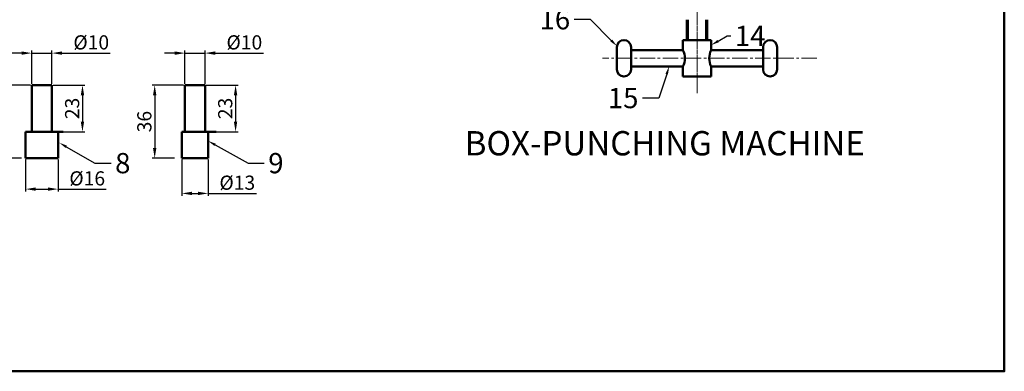
# Model space of a CAD drawing. Units: millimetres. Extents: x 434 to 1535, y -197 to 318.
# Tile 8 of 9: x 1049 to 1535, y -197 to -24. Entities that reach past the tile are written whole.
import ezdxf
from ezdxf import colors
from ezdxf.entities.mleader import LeaderData, LeaderLine
from ezdxf.math import Vec2, Vec3

# ---------------------------------------------------------------- set-up
doc = ezdxf.new("R2010")
doc.units = ezdxf.units.MM
doc.header["$LTSCALE"] = 0.4
doc.linetypes.add('CENTER2', pattern=[28.575, 19.05, -3.175, 3.175, -3.175])
for name, color, linetype, lineweight in [('M-CNTR', 1, 'CENTER2', 18), ('M-DIMS', 2, 'Continuous', 25), ('M-OUTL', 7, 'Continuous', 50), ('M-TEXT', 3, 'Continuous', 25)]:
    doc.layers.add(name, color=color, linetype=linetype, lineweight=lineweight)
doc.styles.get("Standard").update_dxf_attribs({"font": 'arial.ttf'})
doc.dimstyles.new('ISO-25', dxfattribs={"dimtxt": 7, "dimasz": 5, "dimexe": 1.25, "dimexo": 0.625, "dimtad": 1, "dimtoh": 1, "dimdec": 0, "dimtxsty": 'Standard', "dimcen": 2.5, "dimadec": 0, "dimazin": 0, "dimtfac": 1, "dimtdec": 0, "dimtmove": 0, "dimatfit": 3, "dimfxl": 1, "dimarcsym": 0})

# ---------------------------------------------------------------- blocks, each defined once
blk = doc.blocks.new('*U4')
at = {"layer": 'M-CNTR', "color": 0, "transparency": 16777216}
for p, q in [((0, 7), (0, 38.5)), ((-38.5, 0), (-7, 0)), ((7, 0), (73.2, 0)), ((0, -198.75), (0, -7))]:
    blk.add_line(p, q, dxfattribs=at)
at = {"layer": 'M-CNTR', "color": 0, "linetype": 'Continuous', "transparency": 16777216}
for p, q in [((-3.5, 0), (3.5, 0)), ((0, -3.5), (0, 3.5))]:
    blk.add_line(p, q, dxfattribs=at)
blk = doc.blocks.new('*U80')
at = {"layer": 'M-CNTR', "color": 0, "transparency": 16777216}
blk.add_line((0, -17.2), (0, 69.52), dxfattribs=at)
blk = doc.blocks.new('*U81')
at = {"layer": 'M-CNTR', "color": 0, "transparency": 16777216}
blk.add_line((59.26, 0), (-46.77, 0), dxfattribs=at)
blk = doc.blocks.new('*D120')
at = {"layer": 'Defpoints', "color": 0, "ltscale": 0.4, "transparency": 16777216}
for p in [(1064.56, -40.42), (1054.56, -56.24), (1064.56, -56.24)]:
    blk.add_point(p, dxfattribs=at)
at = {"layer": 'M-DIMS', "color": 0, "lineweight": -2, "ltscale": 0.4, "transparency": 16777216}
for p, q in [((1049.56, -40.42), (1044.56, -40.42)), ((1054.56, -55.61), (1054.56, -39.17)), ((1054.56, -40.42), (1064.56, -40.42)), ((1064.56, -55.61), (1064.56, -39.17)), ((1069.56, -40.42), (1093.43, -40.42))]:
    blk.add_line(p, q, dxfattribs=at)
at = {"layer": 'M-DIMS', "color": 0, "ltscale": 0.4, "transparency": 16777216}
for points in [[(1049.56, -39.59), (1049.56, -41.26), (1054.56, -40.42)], [(1069.56, -39.59), (1069.56, -41.26), (1064.56, -40.42)]]:
    blk.add_solid(points, dxfattribs=at)
at = {"layer": 'M-DIMS', "color": 0, "ltscale": 0.4, "transparency": 16777216, "insert": (1083.99, -36.03), "char_height": 7, "attachment_point": 5}
blk.add_mtext('%%C10', dxfattribs=at)
blk = doc.blocks.new('*D121')
at = {"layer": 'Defpoints', "color": 0, "ltscale": 0.4, "transparency": 16777216}
for p in [(1064.56, -56.24), (1064.56, -79.24), (1079.65, -79.24)]:
    blk.add_point(p, dxfattribs=at)
at = {"layer": 'M-DIMS', "color": 0, "lineweight": -2, "ltscale": 0.4, "transparency": 16777216}
for p, q in [((1065.18, -56.24), (1080.9, -56.24)), ((1079.65, -61.24), (1079.65, -74.24)), ((1065.18, -79.24), (1080.9, -79.24))]:
    blk.add_line(p, q, dxfattribs=at)
at = {"layer": 'M-DIMS', "color": 0, "ltscale": 0.4, "transparency": 16777216}
for points in [[(1078.82, -61.24), (1080.48, -61.24), (1079.65, -56.24)], [(1078.82, -74.24), (1080.48, -74.24), (1079.65, -79.24)]]:
    blk.add_solid(points, dxfattribs=at)
at = {"layer": 'M-DIMS', "color": 0, "ltscale": 0.4, "transparency": 16777216, "insert": (1075.45, -67.74), "char_height": 7, "attachment_point": 5, "rotation": 90}
blk.add_mtext('23', dxfattribs=at)
blk = doc.blocks.new('*D119')
at = {"layer": 'Defpoints', "color": 0, "ltscale": 0.4, "transparency": 16777216}
for p in [(1054.56, -56.24), (1039.66, -92.24), (1050.06, -92.24)]:
    blk.add_point(p, dxfattribs=at)
at = {"layer": 'M-DIMS', "color": 0, "lineweight": -2, "ltscale": 0.4, "transparency": 16777216}
for p, q in [((1053.93, -56.24), (1038.41, -56.24)), ((1039.66, -61.24), (1039.66, -87.24)), ((1049.43, -92.24), (1038.41, -92.24))]:
    blk.add_line(p, q, dxfattribs=at)
at = {"layer": 'M-DIMS', "color": 0, "ltscale": 0.4, "transparency": 16777216}
for points in [[(1038.83, -61.24), (1040.49, -61.24), (1039.66, -56.24)], [(1038.83, -87.24), (1040.49, -87.24), (1039.66, -92.24)]]:
    blk.add_solid(points, dxfattribs=at)
at = {"layer": 'M-DIMS', "color": 0, "ltscale": 0.4, "transparency": 16777216, "insert": (1035.46, -74.24), "char_height": 7, "attachment_point": 5, "rotation": 90}
blk.add_mtext('36', dxfattribs=at)
blk = doc.blocks.new('*D123')
at = {"layer": 'Defpoints', "color": 0, "ltscale": 0.4, "transparency": 16777216}
for p in [(1140.27, -40.42), (1130.27, -56.24), (1140.27, -56.24)]:
    blk.add_point(p, dxfattribs=at)
at = {"layer": 'M-DIMS', "color": 0, "lineweight": -2, "ltscale": 0.4, "transparency": 16777216}
for p, q in [((1125.27, -40.42), (1120.27, -40.42)), ((1130.27, -55.61), (1130.27, -39.17)), ((1130.27, -40.42), (1140.27, -40.42)), ((1140.27, -55.61), (1140.27, -39.17)), ((1145.27, -40.42), (1169.13, -40.42))]:
    blk.add_line(p, q, dxfattribs=at)
at = {"layer": 'M-DIMS', "color": 0, "ltscale": 0.4, "transparency": 16777216}
for points in [[(1125.27, -39.59), (1125.27, -41.26), (1130.27, -40.42)], [(1145.27, -39.59), (1145.27, -41.26), (1140.27, -40.42)]]:
    blk.add_solid(points, dxfattribs=at)
at = {"layer": 'M-DIMS', "color": 0, "ltscale": 0.4, "transparency": 16777216, "insert": (1159.7, -36.03), "char_height": 7, "attachment_point": 5}
blk.add_mtext('%%C10', dxfattribs=at)
blk = doc.blocks.new('*D124')
at = {"layer": 'Defpoints', "color": 0, "ltscale": 0.4, "transparency": 16777216}
for p in [(1140.27, -56.24), (1140.27, -79.24), (1155.36, -79.24)]:
    blk.add_point(p, dxfattribs=at)
at = {"layer": 'M-DIMS', "color": 0, "lineweight": -2, "ltscale": 0.4, "transparency": 16777216}
for p, q in [((1140.89, -56.24), (1156.61, -56.24)), ((1155.36, -61.24), (1155.36, -74.24)), ((1140.89, -79.24), (1156.61, -79.24))]:
    blk.add_line(p, q, dxfattribs=at)
at = {"layer": 'M-DIMS', "color": 0, "ltscale": 0.4, "transparency": 16777216}
for points in [[(1154.52, -61.24), (1156.19, -61.24), (1155.36, -56.24)], [(1154.52, -74.24), (1156.19, -74.24), (1155.36, -79.24)]]:
    blk.add_solid(points, dxfattribs=at)
at = {"layer": 'M-DIMS', "color": 0, "ltscale": 0.4, "transparency": 16777216, "insert": (1151.15, -67.74), "char_height": 7, "attachment_point": 5, "rotation": 90}
blk.add_mtext('23', dxfattribs=at)
blk = doc.blocks.new('*D122')
at = {"layer": 'Defpoints', "color": 0, "ltscale": 0.4, "transparency": 16777216}
for p in [(1130.27, -56.24), (1115.37, -92.24), (1125.77, -92.24)]:
    blk.add_point(p, dxfattribs=at)
at = {"layer": 'M-DIMS', "color": 0, "lineweight": -2, "ltscale": 0.4, "transparency": 16777216}
for p, q in [((1129.64, -56.24), (1114.12, -56.24)), ((1115.37, -61.24), (1115.37, -87.24)), ((1125.14, -92.24), (1114.12, -92.24))]:
    blk.add_line(p, q, dxfattribs=at)
at = {"layer": 'M-DIMS', "color": 0, "ltscale": 0.4, "transparency": 16777216}
for points in [[(1114.53, -61.24), (1116.2, -61.24), (1115.37, -56.24)], [(1114.53, -87.24), (1116.2, -87.24), (1115.37, -92.24)]]:
    blk.add_solid(points, dxfattribs=at)
at = {"layer": 'M-DIMS', "color": 0, "ltscale": 0.4, "transparency": 16777216, "insert": (1111.16, -74.24), "char_height": 7, "attachment_point": 5, "rotation": 90}
blk.add_mtext('36', dxfattribs=at)
blk = doc.blocks.new('*D125')
at = {"layer": 'Defpoints', "color": 0, "ltscale": 0.4, "transparency": 16777216}
for p in [(1051.56, -92.24), (1067.56, -92.24), (1067.56, -107.55)]:
    blk.add_point(p, dxfattribs=at)
at = {"layer": 'M-DIMS', "color": 0, "lineweight": -2, "ltscale": 0.4, "transparency": 16777216}
for p, q in [((1051.56, -92.86), (1051.56, -108.8)), ((1067.56, -92.86), (1067.56, -108.8)), ((1056.56, -107.55), (1062.56, -107.55)), ((1067.56, -107.55), (1091.45, -107.55))]:
    blk.add_line(p, q, dxfattribs=at)
at = {"layer": 'M-DIMS', "color": 0, "ltscale": 0.4, "transparency": 16777216}
for points in [[(1056.56, -106.72), (1056.56, -108.39), (1051.56, -107.55)], [(1062.56, -106.72), (1062.56, -108.39), (1067.56, -107.55)]]:
    blk.add_solid(points, dxfattribs=at)
at = {"layer": 'M-DIMS', "color": 0, "ltscale": 0.4, "transparency": 16777216, "insert": (1082, -103.16), "char_height": 7, "attachment_point": 5}
blk.add_mtext('%%C16', dxfattribs=at)
blk = doc.blocks.new('*D126')
at = {"layer": 'Defpoints', "color": 0, "ltscale": 0.4, "transparency": 16777216}
for p in [(1128.77, -92.24), (1141.77, -92.24), (1141.77, -109.69)]:
    blk.add_point(p, dxfattribs=at)
at = {"layer": 'M-DIMS', "color": 0, "lineweight": -2, "ltscale": 0.4, "transparency": 16777216}
for p, q in [((1128.77, -92.86), (1128.77, -110.94)), ((1141.77, -92.86), (1141.77, -110.94)), ((1133.77, -109.69), (1136.77, -109.69)), ((1141.77, -109.69), (1165.66, -109.69))]:
    blk.add_line(p, q, dxfattribs=at)
at = {"layer": 'M-DIMS', "color": 0, "ltscale": 0.4, "transparency": 16777216}
for points in [[(1133.77, -108.85), (1133.77, -110.52), (1128.77, -109.69)], [(1136.77, -108.85), (1136.77, -110.52), (1141.77, -109.69)]]:
    blk.add_solid(points, dxfattribs=at)
at = {"layer": 'M-DIMS', "color": 0, "ltscale": 0.4, "transparency": 16777216, "insert": (1156.21, -105.29), "char_height": 7, "attachment_point": 5}
blk.add_mtext('%%C13', dxfattribs=at)
blk = doc.blocks.new('HANDLE-GRIP')
at = {"ltscale": 0.4}
for p, q in [((0, 14.5), (0, 3.5)), ((7, 3.5), (7, 14.5))]:
    blk.add_line(p, q, dxfattribs=at)
for centre, start, end in [((3.5, 14.5), 0, 180), ((3.5, 3.5), 180, 0)]:
    blk.add_arc(centre, 3.5, start, end, dxfattribs=at)

msp = doc.modelspace()

# ---------------------------------------------------------------- linework, layer by layer
at = {"layer": 'M-OUTL', "ltscale": 0.4}
for p, q in [((1378.54, -33.97), (1378.54, -23.94)), ((1379.04, -33.97), (1379.04, -23.94)), ((1388.04, -33.97), (1388.04, -23.94)), ((1388.54, -33.97), (1388.54, -23.94)), ((1376.54, -33.97), (1376.54, -38.97)), ((1390.54, -33.97), (1376.54, -33.97)), ((1390.54, -38.97), (1390.54, -33.97)), ((1376.54, -38.97), (1350.9, -38.97)), ((1350.9, -38.97), (1350.9, -46.97)), ((1390.54, -38.97), (1416.17, -38.97)), ((1416.17, -38.97), (1416.17, -46.97)), ((1376.54, -46.97), (1350.9, -46.97)), ((1376.54, -46.97), (1376.54, -51.97)), ((1390.54, -51.97), (1390.54, -46.97)), ((1390.54, -46.97), (1416.17, -46.97)), ((1376.54, -51.97), (1390.54, -51.97)), ((1064.56, -56.24), (1054.56, -56.24)), ((1054.56, -56.24), (1054.56, -79.24)), ((1064.56, -79.24), (1064.56, -56.24)), ((1140.27, -56.24), (1130.27, -56.24)), ((1130.27, -56.24), (1130.27, -79.24)), ((1140.27, -79.24), (1140.27, -56.24)), ((1070.06, -79.24), (1051.56, -79.24)), ((1051.56, -79.24), (1051.56, -92.24)), ((1067.56, -92.24), (1067.56, -79.24)), ((1145.77, -79.24), (1128.77, -79.24)), ((1128.77, -79.24), (1128.77, -92.24)), ((1141.77, -92.24), (1141.77, -79.24)), ((1051.56, -92.24), (1067.56, -92.24)), ((1128.77, -92.24), (1141.77, -92.24))]:
    msp.add_line(p, q, dxfattribs=at)
msp.add_lwpolyline([(434.2, 318.45), (1535.47, 318.45), (1535.47, -197.48), (434.2, -197.48)], close=True, dxfattribs=at)
for centre, start, end in [((1368.69, -42.97), 332.9936, 27.0064), ((1398.38, -42.97), 152.9936, 207.0064)]:
    msp.add_arc(centre, 8.81, start, end, dxfattribs=at)

# ---------------------------------------------------------------- block references
at = {"layer": 'M-CNTR'}
for name, p in [('*U4', (1383.54, 149.06)), ('*U80', (1383.54, -42.97)), ('*U81', (1383.54, -42.97))]:
    msp.add_blockref(name, p, dxfattribs=at)
at = {"layer": 'M-OUTL', "rotation": 180}
msp.add_blockref('HANDLE-GRIP', (1350.9, -33.97), dxfattribs=at)
at = {"layer": 'M-OUTL'}
msp.add_blockref('HANDLE-GRIP', (1416.17, -51.97), dxfattribs=at)

# ---------------------------------------------------------------- texts
at = {"layer": 'M-TEXT', "ltscale": 0.4, "insert": (1236.52, -78.91), "char_height": 12, "attachment_point": 1}
msp.add_mtext_dynamic_manual_height_columns('\\pxqc;BOX-PUNCHING MACHINE', width=262.0654, gutter_width=12.5, heights=[0], dxfattribs=at)

# ---------------------------------------------------------------- dimensions: what is measured, and where the dimension line sits
at = {"layer": 'M-DIMS', "ltscale": 0.4}
for base, p1, p2, picture, middle in [((1064.56, -40.42), (1054.56, -56.24), (1064.56, -56.24), '*D120', (1083.99, -36.03)), ((1140.27, -40.42), (1130.27, -56.24), (1140.27, -56.24), '*D123', (1159.7, -36.03))]:
    dim = msp.add_linear_dim(base=base, p1=p1, p2=p2, text='%%C<>', dimstyle='ISO-25', override={"dimclrd": 0, "dimclre": 0, "dimclrt": 0}, dxfattribs=at)
    dim.commit()
    dim.dimension.update_dxf_attribs({"geometry": picture, "text_midpoint": middle})
for base, p1, p2, picture, middle in [((1039.66, -92.24), (1054.56, -56.24), (1050.06, -92.24), '*D119', (1035.46, -74.24)), ((1079.65, -79.24), (1064.56, -56.24), (1064.56, -79.24), '*D121', (1075.45, -67.74)), ((1115.37, -92.24), (1130.27, -56.24), (1125.77, -92.24), '*D122', (1111.16, -74.24)), ((1155.36, -79.24), (1140.27, -56.24), (1140.27, -79.24), '*D124', (1151.15, -67.74))]:
    dim = msp.add_linear_dim(base=base, p1=p1, p2=p2, angle=90, dimstyle='ISO-25', override={"dimclrd": 0, "dimclre": 0, "dimclrt": 0}, dxfattribs=at)
    dim.commit()
    dim.dimension.update_dxf_attribs({"geometry": picture, "text_midpoint": middle})
for base, p1, p2, picture, middle in [((1067.56, -107.55), (1051.56, -92.24), (1067.56, -92.24), '*D125', (1082, -107.55)), ((1141.77, -109.69), (1128.77, -92.24), (1141.77, -92.24), '*D126', (1156.21, -109.69))]:
    dim = msp.add_linear_dim(base=base, p1=p1, p2=p2, text='%%C<>', dimstyle='ISO-25', override={"dimclrd": 0, "dimclre": 0, "dimclrt": 0}, dxfattribs=at)
    dim.commit()
    dim.dimension.update_dxf_attribs({"geometry": picture, "text_midpoint": middle, "dimtype": 160})

# ---------------------------------------------------------------- leaders
at = {"layer": 'M-TEXT', "ltscale": 0.4}
ml = msp.add_multileader_mtext('Standard', dxfattribs=at)
ml.set_content('16', color=256)
ml.set_leader_properties()
ml.build(insert=Vec2(0, 0))
ctx = ml.context
ctx.base_point, ctx.char_height, ctx.plane_origin = Vec3(1305.43, -23.78), 10, Vec3(1343.94, -37)
ctx.text_align_type = 2
notes = []
notes.append((ctx, [(0, (1, 1, 0), (1330.8, -23.78), (-1, 0), 8, [(0, [(1343.94, -37)], 0, [])])]))
ctx.mtext.insert, ctx.mtext.alignment, ctx.mtext.flow_direction = Vec3(1320.8, -18.7), 3, 5
ml = msp.add_multileader_mtext('Standard', dxfattribs=at)
ml.set_content('14', color=256)
ml.set_leader_properties()
ml.build(insert=Vec2(0, 0))
ctx = ml.context
ctx.base_point, ctx.char_height, ctx.plane_origin = Vec3(1400.21, -31.92), 10, Vec3(1390.54, -36.47)
notes.append((ctx, [(0, (1, 1, 0), (1398.42, -31.92), (1, 0), 1.8, [(0, [(1390.54, -36.47)], 0, [])])]))
ctx.mtext.insert, ctx.mtext.flow_direction = Vec3(1402.21, -26.92), 5
ml = msp.add_multileader_mtext('Standard', dxfattribs=at)
ml.set_content('15', color=256)
ml.set_leader_properties()
ml.build(insert=Vec2(0, 0))
ctx = ml.context
ctx.base_point, ctx.char_height, ctx.plane_origin = Vec3(1339.11, -62.7), 10, Vec3(1376.54, -51.97)
ctx.text_align_type = 2
notes.append((ctx, [(0, (1, 1, 0), (1364.57, -62.7), (-1, 0), 8, [(0, [(1369.78, -46.97)], 0, [])])]))
ctx.mtext.insert, ctx.mtext.alignment, ctx.mtext.flow_direction = Vec3(1354.57, -57.61), 3, 5
ml = msp.add_multileader_mtext('Standard', dxfattribs=at)
ml.set_content('8', color=256)
ml.set_leader_properties()
ml.build(insert=Vec2(0, 0))
ctx = ml.context
ctx.base_point, ctx.char_height, ctx.plane_origin = Vec3(1093.8, -94.83), 10, Vec3(1070.06, -85.74)
notes.append((ctx, [(0, (1, 1, 0), (1085.8, -94.83), (1, 0), 8, [(0, [(1068.18, -84.65)], 0, [])])]))
ctx.mtext.insert, ctx.mtext.flow_direction = Vec3(1095.8, -89.74), 5
ml = msp.add_multileader_mtext('Standard', dxfattribs=at)
ml.set_content('9', color=256)
ml.set_leader_properties()
ml.build(insert=Vec2(0, 0))
ctx = ml.context
ctx.base_point, ctx.char_height, ctx.plane_origin = Vec3(1169.51, -94.83), 10, Vec3(1145.77, -85.74)
notes.append((ctx, [(0, (1, 1, 0), (1161.51, -94.83), (1, 0), 8, [(0, [(1141.77, -83.76)], 0, [])])]))
ctx.mtext.insert, ctx.mtext.flow_direction = Vec3(1171.51, -89.74), 5
for ctx, leaders in notes:
    for number, flags, end, landing, length, lines in leaders:
        leader = LeaderData()
        leader.index, (leader.has_last_leader_line, leader.has_dogleg_vector, leader.attachment_direction) = number, flags
        leader.last_leader_point, leader.dogleg_vector, leader.dogleg_length = Vec3(end), Vec3(landing), length
        for number, points, colour, breaks in lines:
            line = LeaderLine()
            line.index, line.vertices, line.color, line.breaks = number, Vec3.list(points), colors.encode_raw_color(colour), breaks
            leader.lines.append(line)
        ctx.leaders.append(leader)

doc.saveas('drawing.dxf')
